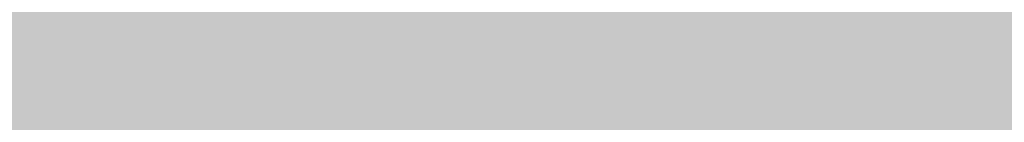
# Model space of a CAD drawing. Units: feet. Extents: x 3168 to 4724, y 827 to 1477.
# Tile 158 of 256: x 3301.2657 to 3301.4016, y 1099.0007 to 1099.0148. Entities that reach past the tile are written whole.
import ezdxf

# ---------------------------------------------------------------- set-up
doc = ezdxf.new("R2010")
doc.units = ezdxf.units.FT
doc.layers.add('A-ELEV', color=7, linetype='Continuous', lineweight=35)
doc.layers.add('A-ELEV-PATT', color=8, linetype='Continuous', lineweight=13)

msp = doc.modelspace()

# ---------------------------------------------------------------- hatches: boundary and pattern name
at = {"layer": 'A-ELEV-PATT'}
h = msp.add_hatch(color=256, dxfattribs=at)
h.dxf.hatch_style = 1
edge = h.paths.add_edge_path()
edge.add_ellipse((3552.90576, 979.22014), major_axis=(36.74492, 0), ratio=0.48484848, start_angle=0, end_angle=360)
edge = h.paths.add_edge_path()
edge.add_ellipse((3559.89164, 929.25228), major_axis=(36.74492, 0), ratio=0.48484848, start_angle=0, end_angle=360)
edge = h.paths.add_edge_path()
edge.add_line((3299.31681, 1198.60608), (3479.91671, 1198.60608))
edge.add_line((3479.91671, 1198.60608), (3479.91671, 1209.86857))
edge.add_spline(control_points=[(3479.91671, 1209.86857), (3464.30116, 1209.86857), (3448.6856, 1209.86857), (3410.94914, 1209.86857), (3388.82823, 1209.86857), (3355.64688, 1209.86857), (3344.58642, 1209.86857), (3327.99574, 1209.86857), (3322.46552, 1209.86857), (3314.17018, 1209.86857), (3311.40507, 1209.86857), (3307.2574, 1209.86857), (3305.87484, 1209.86857), (3303.801, 1209.86857), (3303.10973, 1209.86857), (3302.07281, 1209.86857), (3301.72717, 1209.86857), (3301.20871, 1209.86857), (3301.03589, 1209.86857), (3300.77666, 1209.86857), (3300.69025, 1209.86857), (3300.56064, 1209.86857), (3300.51743, 1209.86857), (3300.45263, 1209.86857), (3300.43102, 1209.86857), (3300.39862, 1209.86857), (3300.38782, 1209.86857), (3300.36622, 1209.86857), (3300.34568, 1209.86857), (3300.34555, 1209.86857), (3300.3455, 1209.86857), (3300.3433, 1209.86857), (3300.34115, 1209.86857), (3300.33791, 1209.86857), (3300.33683, 1209.86857), (3300.33394, 1209.86857), (3300.33213, 1209.86857), (3300.32552, 1209.86858), (3300.32071, 1209.86858), (3300.31092, 1209.86859), (3300.30595, 1209.8686), (3300.29051, 1209.86862), (3300.28005, 1209.86865), (3300.23243, 1209.86878), (3300.1953, 1209.86895), (3299.95107, 1209.87061), (3299.74482, 1209.87433), (3299.43683, 1209.88326), (3299.33439, 1209.88679), (3299.18108, 1209.89292), (3299.13003, 1209.8951), (3298.65222, 1209.9168), (3298.22946, 1209.94572), (3297.60163, 1210.00237), (3297.3934, 1210.02346), (3297.08265, 1210.05831), (3296.97933, 1210.07046), (3296.29295, 1210.15486), (3295.71815, 1210.24336), (3294.86872, 1210.39885), (3294.5877, 1210.45448), (3294.16934, 1210.54335), (3294.03042, 1210.57388), (3291.70715, 1211.1012), (3289.65359, 1211.81344), (3285.77626, 1213.56399), (3283.95141, 1214.60348), (3280.51216, 1216.98008), (3278.89724, 1218.31759), (3276.37991, 1220.82949), (3275.41604, 1221.91774), (3274.03934, 1223.7077), (3273.58104, 1224.34953), (3273.14323, 1225.01632)], knot_values=[39.119033, 39.119033, 39.119033, 39.119033, 39.286353, 39.286353, 39.523379, 39.523379, 39.641892, 39.641892, 39.701148, 39.701148, 39.730777, 39.730777, 39.745591, 39.745591, 39.752998, 39.752998, 39.756701, 39.756701, 39.758553, 39.758553, 39.759479, 39.759479, 39.759942, 39.759942, 39.760173, 39.760173, 39.760289, 39.760289, 39.760405, 39.760405, 39.760463, 39.760463, 39.763389, 39.763389, 39.764851, 39.764851, 39.767304, 39.767304, 39.773825, 39.773825, 39.78057, 39.78057, 39.79477, 39.79477, 39.845194, 39.845194, 40.126715, 40.126715, 40.267476, 40.267476, 40.337856, 40.337856, 40.927023, 40.927023, 41.221606, 41.221606, 41.368898, 41.368898, 42.202622, 42.202622, 42.619485, 42.619485, 42.827916, 42.827916, 46.118323, 46.118323, 49.408731, 49.408731, 52.699139, 52.699139, 54.927489, 54.927489, 56.104228, 56.104228, 56.104228, 56.104228], weights=[1, 1, 1, 1, 1, 1, 1, 1, 1, 1, 1, 1, 1, 1, 1, 1, 1, 1, 1, 1, 1, 1, 1, 1, 1, 1, 1, 1, 1, 1, 1, 1, 1, 1, 1, 1, 1, 1, 1, 1, 1, 1, 1, 1, 1, 1, 1, 1, 1, 1, 1, 1, 1, 1, 1, 1, 1, 1, 1, 1, 1, 1, 1, 1, 1, 1, 1, 1, 1, 1, 1, 1, 1, 1], degree=3, periodic=0)
edge.add_line((3273.14323, 1225.01632), (3273.14323, 1099.01632))
edge.add_line((3273.14323, 1099.01632), (3299.31681, 1099.01632))
edge.add_line((3299.31681, 1099.01632), (3299.31681, 1198.60608))
edge = h.paths.add_edge_path()
edge.add_line((3304.75844, 1324.15806), (3479.91671, 1324.15806))
edge.add_line((3479.91671, 1324.15806), (3479.91671, 1335.71462))
edge.add_line((3479.91671, 1335.71462), (3269.16163, 1335.71462))
edge.add_spline(control_points=[(3269.16163, 1335.71462), (3264.02423, 1335.71462), (3258.36412, 1328.95819), (3259.26431, 1323.90027)], knot_values=[0, 0, 0, 0, 15.412191, 15.412191, 15.412191, 15.412191], degree=3, periodic=0)
edge.add_line((3259.26431, 1323.90027), (3265.51685, 1288.76913))
edge.add_line((3265.51685, 1288.76913), (3275.2651, 1261.54563))
edge.add_line((3275.2651, 1261.54563), (3304.75844, 1261.54563))
edge.add_line((3304.75844, 1261.54563), (3304.75844, 1324.15806))
h = msp.add_hatch(color=256, dxfattribs=at)
h.dxf.hatch_style = 1
h.paths.add_polyline_path([(3384.52525, 1099.01632), (3335.02917, 1099.01632), (3299.31681, 1099.01632), (3273.14323, 1099.01632), (3217.56536, 1099.01632), (3168.06928, 827.11626), (3335.02917, 827.11626)])

# ---------------------------------------------------------------- linework, layer by layer
at = {"layer": 'A-ELEV'}
msp.add_open_spline([(3808.5202, 1099.01632), (3808.5202, 1141.41324), (3808.5202, 1183.81015), (3808.5202, 1226.63532), (3808.5202, 1227.06358), (3808.5202, 1227.49183), (3811.49187, 1248.99467), (3814.46354, 1270.49752), (3817.46523, 1292.21756), (3817.49525, 1292.43476), (3817.52526, 1292.65196), (3817.5728, 1310.10675), (3817.62034, 1327.56153), (3817.66788, 1345.01632), (3817.66788, 1345.45796), (3817.66788, 1345.89961), (3817.66788, 1346.45605), (3817.66788, 1346.57084), (3817.66788, 1346.75289), (3817.66788, 1346.82014), (3817.66788, 1346.93487), (3817.66788, 1346.98234), (3817.66788, 1347.03859), (3817.66788, 1347.04736), (3817.66788, 1347.07366), (3817.66788, 1347.0593), (3817.66788, 1347.06155), (3817.66788, 1347.06267), (3817.66788, 1347.06603), (3817.66787, 1347.06827), (3817.66787, 1347.075), (3817.66787, 1347.07949), (3817.66785, 1347.09294), (3817.66783, 1347.1019), (3817.66777, 1347.12879), (3817.6677, 1347.1467), (3817.66743, 1347.20042), (3817.66716, 1347.23619), (3817.6661, 1347.34338), (3817.66504, 1347.41469), (3817.66081, 1347.62809), (3817.65661, 1347.76971), (3817.63997, 1348.19249), (3817.62351, 1348.47159), (3817.55909, 1349.30007), (3817.49612, 1349.84059), (3817.25543, 1351.42416), (3817.02632, 1352.42879), (3816.30687, 1354.88891), (3815.74375, 1356.26873), (3814.46396, 1358.81921), (3813.74641, 1359.99097), (3812.19584, 1362.17234), (3811.36225, 1363.18212), (3809.58884, 1365.06901), (3808.64882, 1365.94611), (3806.65426, 1367.57962), (3805.5997, 1368.33615), (3803.35289, 1369.72233), (3802.16054, 1370.35239), (3799.60081, 1371.45359), (3798.23269, 1371.92548), (3795.28008, 1372.63462), (3793.69315, 1372.87207), (3791.86944, 1372.92648), (3791.74086, 1372.92922), (3791.35337, 1372.9341), (3791.09271, 1372.9329), (3790.30412, 1372.91507), (3789.76954, 1372.88419), (3789.20919, 1372.83024), (3789.19062, 1372.82842), (3789.13489, 1372.82291), (3789.0977, 1372.81914), (3789.04844, 1372.81401), (3789.0364, 1372.81274), (3789.00026, 1372.80892), (3788.97615, 1372.80633), (3788.9494, 1372.8034), (3788.94679, 1372.80312), (3788.94257, 1372.80266), (3788.94097, 1372.80248), (3788.93857, 1372.80222), (3788.93778, 1372.80213), (3788.93539, 1372.80187), (3788.86753, 1372.7944), (3788.75687, 1372.78223), (3788.70153, 1372.77614), (3788.53553, 1372.75788), (3788.42486, 1372.74571), (3788.09286, 1372.70918), (3787.87152, 1372.68484), (3787.20751, 1372.61179), (3786.76483, 1372.5631), (3785.43681, 1372.41701), (3784.55147, 1372.31962), (3781.89542, 1372.02744), (3780.12473, 1371.83266), (3774.81265, 1371.24831), (3771.27126, 1370.85874), (3760.64709, 1369.69004), (3753.56431, 1368.9109), (3732.31597, 1366.5735), (3718.15042, 1365.01523), (3694.00676, 1362.35933), (3684.02866, 1361.26169), (3674.05056, 1360.16406), (3664.60066, 1360.16406), (3655.15077, 1360.16406), (3626.80108, 1360.16406), (3607.90129, 1360.16406), (3551.20192, 1360.16406), (3513.40234, 1360.16406), (3467.72518, 1360.16406), (3459.8476, 1360.16406), (3436.21487, 1360.16406), (3420.45972, 1360.16406), (3373.19425, 1360.16406), (3341.68395, 1360.16406), (3302.84816, 1360.16406), (3295.52269, 1360.16406), (3286.03829, 1360.16406), (3283.87937, 1360.16406), (3277.40261, 1360.16406), (3273.08477, 1360.16406), (3267.73285, 1360.16406), (3266.69877, 1360.16406), (3263.59652, 1360.16406), (3261.52835, 1360.16406), (3259.23694, 1360.16406), (3259.0137, 1360.16406), (3258.34396, 1360.16406), (3257.89747, 1360.16406), (3257.431, 1360.16406), (3257.41102, 1360.16406), (3257.37057, 1360.16406), (3257.37547, 1360.16406), (3257.3746, 1360.16406), (3257.37394, 1360.16406), (3257.37196, 1360.16406), (3257.37064, 1360.16406), (3257.36667, 1360.16406), (3257.36403, 1360.16406), (3257.35611, 1360.16405), (3257.35083, 1360.16405), (3257.33499, 1360.16402), (3257.32443, 1360.164), (3257.29277, 1360.1639), (3257.27168, 1360.1638), (3257.20844, 1360.1634), (3257.16634, 1360.163), (3257.04021, 1360.16139), (3256.95635, 1360.15978), (3256.7055, 1360.15339), (3256.53924, 1360.14704), (3256.04357, 1360.12192), (3255.7173, 1360.0971), (3254.75245, 1360.00048), (3254.12797, 1359.90651), (3252.18007, 1359.52533), (3250.94157, 1359.14399), (3248.67018, 1358.24329), (3247.63574, 1357.72383), (3245.73263, 1356.60347), (3244.86339, 1356.00206), (3243.25311, 1354.74287), (3242.51197, 1354.08473), (3240.75105, 1352.34478), (3239.80096, 1351.22957), (3238.08777, 1348.87244), (3237.32469, 1347.63036), (3235.98251, 1344.97163), (3235.40221, 1343.55491), (3234.59108, 1340.81546), (3234.31088, 1339.54355), (3233.97649, 1336.80256), (3233.92211, 1335.33088), (3234.14892, 1332.59127), (3234.34953, 1331.3672), (3234.71989, 1329.99937), (3234.75242, 1329.88336), (3234.85362, 1329.5348), (3234.92589, 1329.30168), (3235.02484, 1329.00255), (3235.04692, 1328.93693), (3235.07764, 1328.84724), (3235.08592, 1328.8232), (3235.11094, 1328.75106), (3235.12783, 1328.70296), (3235.14799, 1328.64624), (3235.15106, 1328.63763), (3235.1561, 1328.62353), (3235.15806, 1328.61803), (3235.16021, 1328.61203), (3235.16561, 1328.59694), (3235.1801, 1328.55649), (3235.19026, 1328.5281), (3235.22076, 1328.44295), (3235.24108, 1328.38618), (3235.30207, 1328.21587), (3235.34273, 1328.10232), (3235.4647, 1327.7617), (3235.54601, 1327.53462), (3235.78995, 1326.85338), (3235.95258, 1326.39922), (3236.44046, 1325.03674), (3236.76571, 1324.12841), (3237.74148, 1321.40345), (3238.39198, 1319.5868), (3240.34351, 1314.13687), (3241.64452, 1310.50358), (3245.54757, 1299.60371), (3248.14961, 1292.33713), (3255.95571, 1270.53739), (3261.15977, 1256.00423), (3267.38762, 1238.612), (3268.4114, 1235.75294), (3269.51038, 1232.68386), (3269.58558, 1232.47385), (3269.70661, 1232.13585), (3269.75244, 1232.00786), (3269.82733, 1231.79873), (3269.85638, 1231.7176), (3269.90632, 1231.57812), (3269.92721, 1231.51978), (3269.97247, 1231.39341), (3269.99683, 1231.32537), (3270.0265, 1231.24251), (3270.03181, 1231.22768), (3270.04028, 1231.20402), (3270.03922, 1231.20698), (3270.03936, 1231.2066), (3270.03943, 1231.20641), (3270.03963, 1231.20585), (3270.03977, 1231.20547), (3270.04017, 1231.20433), (3270.04044, 1231.20358), (3270.04125, 1231.20131), (3270.0418, 1231.1998), (3270.04342, 1231.19527), (3270.0445, 1231.19225), (3270.04776, 1231.18318), (3270.04993, 1231.17714), (3270.05644, 1231.15903), (3270.06079, 1231.14696), (3270.07387, 1231.11076), (3270.08261, 1231.08666), (3270.10894, 1231.01441), (3270.1266, 1230.96635), (3270.17993, 1230.82246), (3270.21595, 1230.72692), (3270.32532, 1230.44151), (3270.40003, 1230.25281), (3270.62925, 1229.69144), (3270.78888, 1229.3235), (3271.28649, 1228.23832), (3271.6431, 1227.53975), (3272.77586, 1225.51528), (3273.61417, 1224.2605), (3275.41604, 1221.91774), (3276.37991, 1220.82949), (3278.89724, 1218.31759), (3280.51216, 1216.98008), (3283.95141, 1214.60348), (3285.77626, 1213.56399), (3289.65359, 1211.81344), (3291.70715, 1211.1012), (3294.03042, 1210.57388), (3294.16934, 1210.54335), (3294.5877, 1210.45448), (3294.86872, 1210.39885), (3295.71815, 1210.24336), (3296.29295, 1210.15486), (3296.97933, 1210.07046), (3297.08265, 1210.05831), (3297.3934, 1210.02346), (3297.60163, 1210.00237), (3298.22946, 1209.94572), (3298.65222, 1209.9168), (3299.13003, 1209.8951), (3299.18108, 1209.89292), (3299.33439, 1209.88679), (3299.43683, 1209.88326), (3299.74482, 1209.87433), (3299.95107, 1209.87061), (3300.1953, 1209.86895), (3300.23243, 1209.86878), (3300.28005, 1209.86865), (3300.29051, 1209.86862), (3300.30595, 1209.8686), (3300.31092, 1209.86859), (3300.32071, 1209.86858), (3300.32552, 1209.86858), (3300.33213, 1209.86857), (3300.33394, 1209.86857), (3300.33683, 1209.86857), (3300.33791, 1209.86857), (3300.34115, 1209.86857), (3300.3433, 1209.86857), (3300.3455, 1209.86857), (3300.34555, 1209.86857), (3300.34568, 1209.86857), (3300.36622, 1209.86857), (3300.38782, 1209.86857), (3300.39862, 1209.86857), (3300.43102, 1209.86857), (3300.45263, 1209.86857), (3300.51743, 1209.86857), (3300.56064, 1209.86857), (3300.69025, 1209.86857), (3300.77666, 1209.86857), (3301.03589, 1209.86857), (3301.20871, 1209.86857), (3301.72717, 1209.86857), (3302.07281, 1209.86857), (3303.10973, 1209.86857), (3303.801, 1209.86857), (3305.87484, 1209.86857), (3307.2574, 1209.86857), (3311.40507, 1209.86857), (3314.17018, 1209.86857), (3322.46552, 1209.86857), (3327.99574, 1209.86857), (3344.58642, 1209.86857), (3355.64688, 1209.86857), (3388.82823, 1209.86857), (3410.94914, 1209.86857), (3477.31185, 1209.86857), (3521.55366, 1209.86857), (3566.83618, 1209.86857), (3567.87689, 1209.86857), (3570.99902, 1209.86857), (3573.08043, 1209.86857), (3575.7814, 1209.86857), (3576.40094, 1209.86857), (3577.29582, 1209.86857), (3577.57115, 1209.86857), (3578.39715, 1209.86857), (3578.94781, 1209.86857), (3579.75649, 1209.86857), (3580.01451, 1209.86857), (3580.34274, 1209.86857), (3580.32686, 1209.86857), (3580.32717, 1209.86857), (3580.32732, 1209.86857), (3580.32778, 1209.86857), (3580.32809, 1209.86857), (3580.329, 1209.86857), (3580.32961, 1209.86857), (3580.33145, 1209.86857), (3580.33267, 1209.86857), (3580.33633, 1209.86857), (3580.33878, 1209.86857), (3580.34611, 1209.86856), (3580.35099, 1209.86856), (3580.36566, 1209.86854), (3580.37544, 1209.86852), (3580.4048, 1209.86845), (3580.42439, 1209.86838), (3580.48318, 1209.86808), (3580.52244, 1209.86779), (3580.64036, 1209.86662), (3580.71919, 1209.86545), (3580.95632, 1209.86077), (3581.11522, 1209.85607), (3581.59416, 1209.83723), (3581.91642, 1209.81833), (3582.88995, 1209.74243), (3583.54799, 1209.66617), (3585.53183, 1209.36062), (3586.86722, 1209.05389), (3589.47155, 1208.25247), (3590.74024, 1207.75785), (3591.99545, 1207.1588), (3592.05781, 1207.12874), (3592.24424, 1207.03795), (3592.36768, 1206.97663), (3592.73528, 1206.79036), (3592.97675, 1206.6631), (3593.24454, 1206.51644), (3593.27473, 1206.49982), (3593.36512, 1206.44984), (3593.42511, 1206.41633), (3593.60431, 1206.31529), (3593.72273, 1206.24721), (3593.85721, 1206.1684), (3593.87436, 1206.15832), (3593.92574, 1206.12804), (3593.9599, 1206.1078), (3594.06209, 1206.0469), (3594.12983, 1206.00607), (3594.20844, 1205.95817), (3594.21968, 1205.9513), (3594.25339, 1205.93069), (3594.27582, 1205.91692), (3594.34297, 1205.87554), (3594.38756, 1205.84785), (3594.43362, 1205.81905), (3594.43526, 1205.81802), (3594.44017, 1205.81495), (3594.44345, 1205.81289), (3594.44712, 1205.81059), (3594.44752, 1205.81035), (3594.44869, 1205.80961), (3594.44948, 1205.80912), (3594.45037, 1205.80856), (3594.45047, 1205.8085), (3594.4506, 1205.80842), (3594.4674, 1205.79789), (3594.49327, 1205.78167), (3594.5062, 1205.77357), (3594.54501, 1205.74925), (3594.57088, 1205.73303), (3594.64849, 1205.6844), (3594.70023, 1205.65197), (3594.85544, 1205.55469), (3594.95892, 1205.48984), (3595.26936, 1205.29528), (3595.47631, 1205.16558), (3596.09719, 1204.77646), (3596.5111, 1204.51705), (3597.75284, 1203.73883), (3598.58067, 1203.22001), (3601.06415, 1201.66355), (3602.71981, 1200.62591), (3607.68677, 1197.513), (3610.99809, 1195.43773), (3620.93202, 1189.2119), (3627.55464, 1185.06135), (3647.42251, 1172.60971), (3660.66775, 1164.30861), (3700.40348, 1139.40531), (3726.89397, 1122.80312), (3757.20572, 1103.80605), (3761.02697, 1101.41118), (3764.84822, 1099.01632), (3745.32827, 1099.01632), (3725.80832, 1099.01632), (3706.28837, 1099.01632), (3706.28837, 1108.45324), (3706.28837, 1117.89016), (3706.28837, 1127.32708), (3710.75075, 1127.32708), (3715.21314, 1127.32708), (3719.67553, 1127.32708)], degree=3, knots=[0, 0, 0, 0, 0.982037, 0.982037, 0.991957, 0.991957, 0.991957, 1.966522, 1.966522, 1.976367, 1.976367, 1.976367, 2.976367, 2.976367, 2.976367, 3.00169, 3.00169, 3.008272, 3.008272, 3.012129, 3.012129, 3.014851, 3.014851, 3.015353, 3.015353, 3.016359, 3.016359, 3.017365, 3.017365, 3.019376, 3.019376, 3.023398, 3.023398, 3.031442, 3.031442, 3.047531, 3.047531, 3.079708, 3.079708, 3.144063, 3.144063, 3.272772, 3.272772, 3.53019, 3.53019, 4.045026, 4.045026, 5.074698, 5.074698, 6.700878, 6.700878, 8.327058, 8.327058, 9.953238, 9.953238, 11.579418, 11.579418, 13.205598, 13.205598, 14.831778, 14.831778, 16.457958, 16.457958, 18.084138, 18.084138, 18.206872, 18.206872, 18.45234, 18.45234, 18.943275, 18.943275, 18.960093, 18.960093, 18.993729, 18.993729, 19.00461, 19.00461, 19.026374, 19.026374, 19.028737, 19.028737, 19.03018, 19.03018, 19.030897, 19.030897, 19.032332, 19.032332, 19.033766, 19.033766, 19.036636, 19.036636, 19.042374, 19.042374, 19.053851, 19.053851, 19.076805, 19.076805, 19.122714, 19.122714, 19.21453, 19.21453, 19.398163, 19.398163, 19.765429, 19.765429, 20.024128, 20.024128, 20.024128, 20.092031, 20.092031, 20.227836, 20.227836, 20.499446, 20.499446, 20.556051, 20.556051, 20.66926, 20.66926, 20.895678, 20.895678, 20.948316, 20.948316, 20.963829, 20.963829, 20.994855, 20.994855, 21.002285, 21.002285, 21.017146, 21.017146, 21.01875, 21.01875, 21.021959, 21.021959, 21.022102, 21.022102, 21.022249, 21.022249, 21.022708, 21.022708, 21.023627, 21.023627, 21.025464, 21.025464, 21.029138, 21.029138, 21.036486, 21.036486, 21.051183, 21.051183, 21.080575, 21.080575, 21.139361, 21.139361, 21.256932, 21.256932, 21.492073, 21.492073, 21.962356, 21.962356, 23.01002, 23.01002, 24.057684, 24.057684, 25.105348, 25.105348, 26.153011, 26.153011, 27.776787, 27.776787, 29.400562, 29.400562, 31.024337, 31.024337, 32.278801, 32.278801, 33.533265, 33.533265, 34.467568, 34.467568, 34.553971, 34.553971, 34.726776, 34.726776, 34.775309, 34.775309, 34.793079, 34.793079, 34.82862, 34.82862, 34.834979, 34.834979, 34.839039, 34.839039, 34.839411, 34.839411, 34.840285, 34.840285, 34.842034, 34.842034, 34.845531, 34.845531, 34.852525, 34.852525, 34.866512, 34.866512, 34.894488, 34.894488, 34.950439, 34.950439, 35.062342, 35.062342, 35.286147, 35.286147, 35.733758, 35.733758, 35.821815, 35.821815, 35.828283, 35.828283, 35.832225, 35.832225, 35.834724, 35.834724, 35.836521, 35.836521, 35.838617, 35.838617, 35.839073, 35.839073, 35.839345, 35.839345, 35.839617, 35.839617, 35.840161, 35.840161, 35.841249, 35.841249, 35.843425, 35.843425, 35.847778, 35.847778, 35.856482, 35.856482, 35.873891, 35.873891, 35.908709, 35.908709, 35.978345, 35.978345, 36.117617, 36.117617, 36.396161, 36.396161, 36.953248, 36.953248, 38.067423, 38.067423, 40.295772, 40.295772, 42.524122, 42.524122, 45.81453, 45.81453, 49.104937, 49.104937, 52.395345, 52.395345, 52.603776, 52.603776, 53.020639, 53.020639, 53.854363, 53.854363, 54.001655, 54.001655, 54.296238, 54.296238, 54.885405, 54.885405, 54.955785, 54.955785, 55.096546, 55.096546, 55.378067, 55.378067, 55.42849, 55.42849, 55.442691, 55.442691, 55.449436, 55.449436, 55.455957, 55.455957, 55.458409, 55.458409, 55.459872, 55.459872, 55.462798, 55.462798, 55.462856, 55.462856, 55.462972, 55.462972, 55.463088, 55.463088, 55.463319, 55.463319, 55.463782, 55.463782, 55.464708, 55.464708, 55.46656, 55.46656, 55.470263, 55.470263, 55.47767, 55.47767, 55.492484, 55.492484, 55.522112, 55.522112, 55.581369, 55.581369, 55.699882, 55.699882, 55.936907, 55.936907, 56.410959, 56.410959, 56.42211, 56.42211, 56.444413, 56.444413, 56.451051, 56.451051, 56.454001, 56.454001, 56.459901, 56.459901, 56.462666, 56.462666, 56.463418, 56.463418, 56.464171, 56.464171, 56.465675, 56.465675, 56.468684, 56.468684, 56.474702, 56.474702, 56.486738, 56.486738, 56.51081, 56.51081, 56.558955, 56.558955, 56.655243, 56.655243, 56.847821, 56.847821, 57.232975, 57.232975, 58.003284, 58.003284, 59.543901, 59.543901, 62.625137, 62.625137, 68.787607, 68.787607, 74.950078, 74.950078, 75.27336, 75.27336, 75.919923, 75.919923, 77.213051, 77.213051, 77.377769, 77.377769, 77.707206, 77.707206, 78.366079, 78.366079, 78.462532, 78.462532, 78.655436, 78.655436, 79.041245, 79.041245, 79.105735, 79.105735, 79.234714, 79.234714, 79.492672, 79.492672, 79.502197, 79.502197, 79.521249, 79.521249, 79.523534, 79.523534, 79.528103, 79.528103, 79.528682, 79.528682, 79.528885, 79.528885, 79.529089, 79.529089, 79.529495, 79.529495, 79.530308, 79.530308, 79.531935, 79.531935, 79.535187, 79.535187, 79.541693, 79.541693, 79.554704, 79.554704, 79.580725, 79.580725, 79.632769, 79.632769, 79.736856, 79.736856, 79.94503, 79.94503, 80.361377, 80.361377, 80.421435, 80.421435, 80.421435, 81.421435, 81.421435, 81.421435, 82.421435, 82.421435, 82.421435, 83.421435, 83.421435, 83.421435, 83.421435], dxfattribs=at)

doc.saveas('drawing.dxf')
